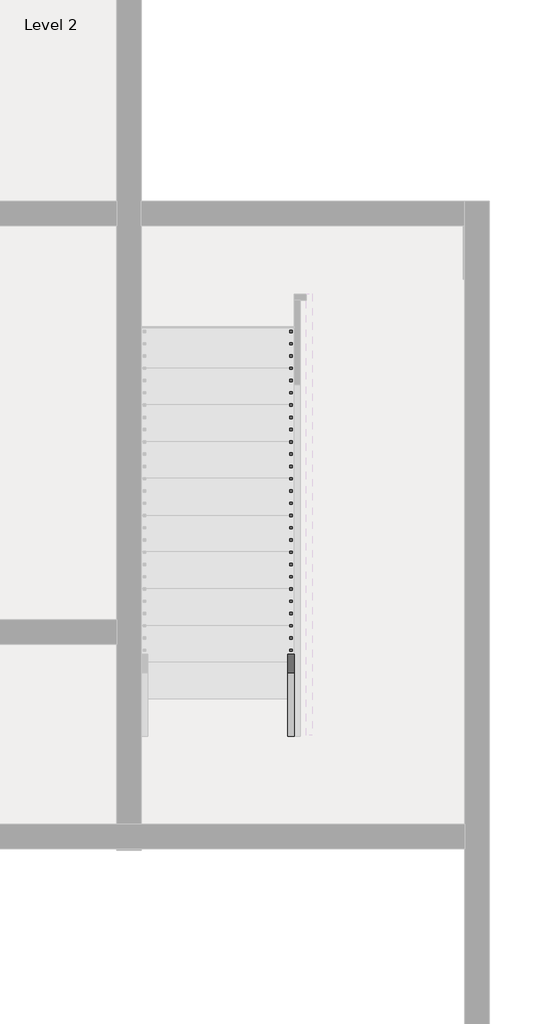
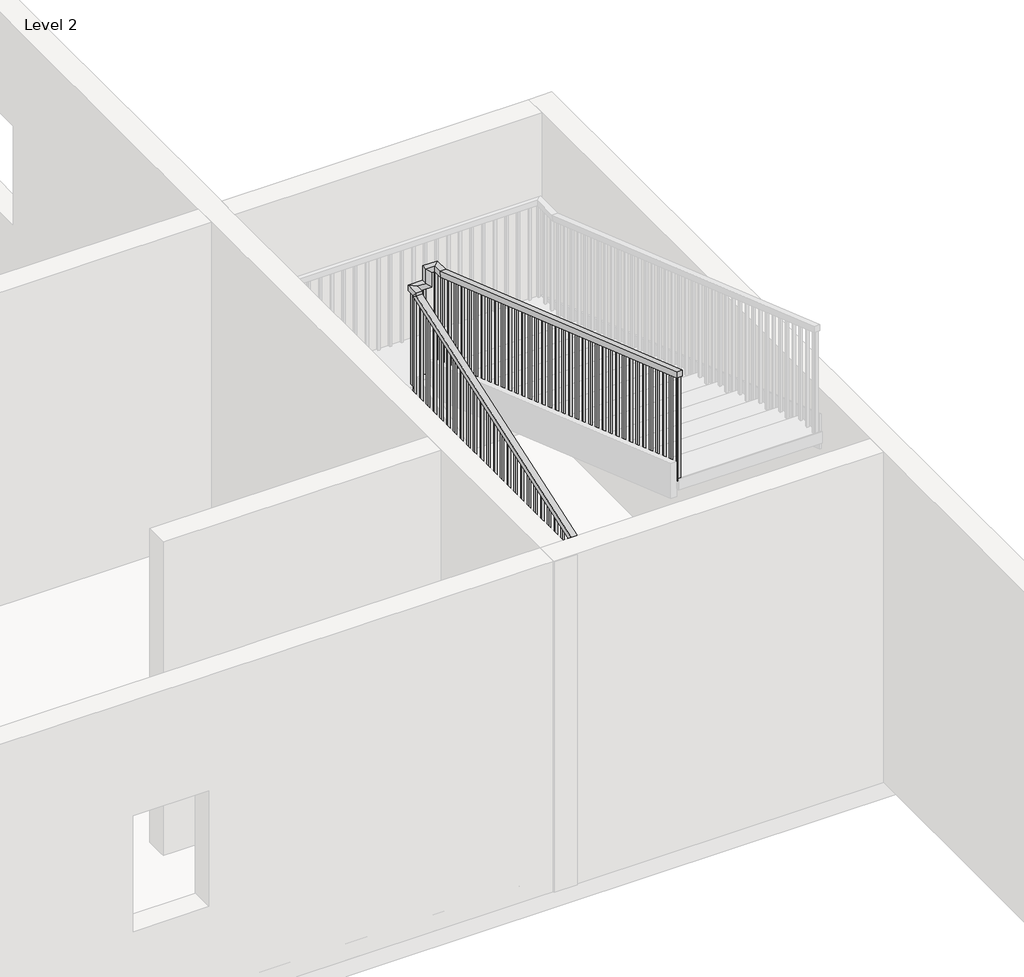
# One storey, part 6 of 14: 1 railing.
"""IFC4 building model written with IfcOpenShell, lengths in millimetres."""

from ifc_helpers import new_model, si_unit, frame, origin, place, context, project, spatial, polyline, outline, extrude, faceted_brep, element, save

model = new_model("IFC4")

# Units and contexts
model_context = context("Model", 3, world=origin())
ifc_project = project(units=[si_unit("LENGTHUNIT", "METRE", prefix="MILLI")], contexts=[model_context])

# Site, building, storey
site = spatial("IfcSite", under=ifc_project)
building = spatial("IfcBuilding", under=site)
storey = spatial("IfcBuildingStorey", under=building, Name="Level 2", Elevation=3048.0)

# Railing
placement = place(None, origin())
element("IfcRailing", 1, ObjectType="Handrail - Rectangular", at=placement, inside=storey, context=model_context, shape_type="SolidModel", body=[
    faceted_brep([(-2644.5381751, -9955.5916506, 4067.9076923), (-2644.5381751, -9955.5916506, 4014.1602476), (-2593.7381751, -9955.5916506, 4014.1602476), (-2593.7381751, -9955.5916506, 4067.9076923), (-2644.5381751, -6367.8416506, 5307.6687908), (-2644.5381751, -6317.0416506, 5271.4754856), (-2593.7381751, -6317.0416506, 5271.4754856), (-2593.7381751, -6367.8416506, 5307.6687908), (-2644.5381751, -6367.8416506, 5334.0), (-2644.5381751, -6317.0416506, 5283.2), (-2593.7381751, -6317.0416506, 5283.2), (-2593.7381751, -6367.8416506, 5334.0), (-2644.5381751, -6240.8416506, 5334.0), (-2644.5381751, -6240.8416506, 5283.2), (-2593.7381751, -6291.6416506, 5283.2), (-2593.7381751, -6291.6416506, 5334.0), (-2517.5381751, -6240.8416506, 5334.0), (-2466.7381751, -6240.8416506, 5283.2), (-2466.7381751, -6291.6416506, 5283.2), (-2517.5381751, -6291.6416506, 5334.0), (-2517.5381751, -6240.8416506, 5465.8846154), (-2466.7381751, -6240.8416506, 5415.0846154), (-2466.7381751, -6291.6416506, 5415.0846154), (-2517.5381751, -6291.6416506, 5465.8846154), (-2390.5381751, -6240.8416506, 5465.8846154), (-2390.5381751, -6240.8416506, 5415.0846154), (-2441.3381751, -6291.6416506, 5415.0846154), (-2441.3381751, -6291.6416506, 5465.8846154), (-2390.5381751, -6367.8416506, 5465.8846154), (-2390.5381751, -6376.3852679, 5415.0846154), (-2441.3381751, -6376.3852679, 5415.0846154), (-2441.3381751, -6367.8416506, 5465.8846154), (-2390.5381751, -9949.2416506, 6705.6), (-2441.3381751, -9949.2416506, 6705.6), (-2441.3381751, -9949.2416506, 6651.842594), (-2390.5381751, -9949.2416506, 6651.842594)], [[[0, 1, 2, 3]], [[1, 0, 4, 5]], [[2, 1, 5, 6]], [[3, 2, 6, 7]], [[0, 3, 7, 4]], [[5, 4, 8, 9]], [[6, 5, 9, 10]], [[7, 6, 10, 11]], [[4, 7, 11, 8]], [[9, 8, 12, 13]], [[10, 9, 13, 14]], [[11, 10, 14, 15]], [[8, 11, 15, 12]], [[13, 12, 16, 17]], [[14, 13, 17, 18]], [[15, 14, 18, 19]], [[12, 15, 19, 16]], [[17, 16, 20, 21]], [[18, 17, 21, 22]], [[19, 18, 22, 23]], [[16, 19, 23, 20]], [[21, 20, 24, 25]], [[22, 21, 25, 26]], [[23, 22, 26, 27]], [[20, 23, 27, 24]], [[25, 24, 28, 29]], [[26, 25, 29, 30]], [[27, 26, 30, 31]], [[24, 27, 31, 28]], [[32, 33, 34, 35]], [[29, 28, 32, 35]], [[30, 29, 35, 34]], [[31, 30, 34, 33]], [[28, 31, 33, 32]]]),
    extrude(outline(polyline([(-9933.3666506, 6646.3474017), (-9914.3166506, 6639.7531709), (-9914.3166506, 5685.6923077), (-9933.3666506, 5685.6923077), (-9933.3666506, 6646.3474017)])), frame((-2425.4631751, 0.0, 0.0), z_axis=(1.0, 0.0, 0.0), x_axis=(0.0, 1.0, 0.0)), (0.0, 0.0, 1.0), 19.05),
    extrude(outline(polyline([(-9831.7666506, 6611.1781709), (-9812.7166506, 6604.5839402), (-9812.7166506, 5685.6923077), (-9831.7666506, 5685.6923077), (-9831.7666506, 6611.1781709)])), frame((-2425.4631751, 0.0, 0.0), z_axis=(1.0, 0.0, 0.0), x_axis=(0.0, 1.0, 0.0)), (0.0, 0.0, 1.0), 19.05),
    extrude(outline(polyline([(-9730.1666506, 6576.0089402), (-9711.1166506, 6569.4147094), (-9711.1166506, 5685.6923077), (-9730.1666506, 5685.6923077), (-9730.1666506, 6576.0089402)])), frame((-2425.4631751, 0.0, 0.0), z_axis=(1.0, 0.0, 0.0), x_axis=(0.0, 1.0, 0.0)), (0.0, 0.0, 1.0), 19.05),
    extrude(outline(polyline([(-9628.5666506, 6540.8397094), (-9609.5166506, 6534.2454786), (-9609.5166506, 5580.1846154), (-9628.5666506, 5580.1846154), (-9628.5666506, 6540.8397094)])), frame((-2425.4631751, 0.0, 0.0), z_axis=(1.0, 0.0, 0.0), x_axis=(0.0, 1.0, 0.0)), (0.0, 0.0, 1.0), 19.05),
    extrude(outline(polyline([(-9526.9666506, 6505.6704786), (-9507.9166506, 6499.0762479), (-9507.9166506, 5580.1846154), (-9526.9666506, 5580.1846154), (-9526.9666506, 6505.6704786)])), frame((-2425.4631751, 0.0, 0.0), z_axis=(1.0, 0.0, 0.0), x_axis=(0.0, 1.0, 0.0)), (0.0, 0.0, 1.0), 19.05),
    extrude(outline(polyline([(-9425.3666506, 6470.5012479), (-9406.3166506, 6463.9070171), (-9406.3166506, 5580.1846154), (-9425.3666506, 5580.1846154), (-9425.3666506, 6470.5012479)])), frame((-2425.4631751, 0.0, 0.0), z_axis=(1.0, 0.0, 0.0), x_axis=(0.0, 1.0, 0.0)), (0.0, 0.0, 1.0), 19.05),
    extrude(outline(polyline([(-9323.7666506, 6435.3320171), (-9304.7166506, 6428.7377863), (-9304.7166506, 5474.6769231), (-9323.7666506, 5474.6769231), (-9323.7666506, 6435.3320171)])), frame((-2425.4631751, 0.0, 0.0), z_axis=(1.0, 0.0, 0.0), x_axis=(0.0, 1.0, 0.0)), (0.0, 0.0, 1.0), 19.05),
    extrude(outline(polyline([(-9222.1666506, 6400.1627863), (-9203.1166506, 6393.5685556), (-9203.1166506, 5474.6769231), (-9222.1666506, 5474.6769231), (-9222.1666506, 6400.1627863)])), frame((-2425.4631751, 0.0, 0.0), z_axis=(1.0, 0.0, 0.0), x_axis=(0.0, 1.0, 0.0)), (0.0, 0.0, 1.0), 19.05),
    extrude(outline(polyline([(-9120.5666506, 6364.9935556), (-9101.5166506, 6358.3993248), (-9101.5166506, 5474.6769231), (-9120.5666506, 5474.6769231), (-9120.5666506, 6364.9935556)])), frame((-2425.4631751, 0.0, 0.0), z_axis=(1.0, 0.0, 0.0), x_axis=(0.0, 1.0, 0.0)), (0.0, 0.0, 1.0), 19.05),
    extrude(outline(polyline([(-9018.9666506, 6329.8243248), (-8999.9166506, 6323.230094), (-8999.9166506, 5369.1692308), (-9018.9666506, 5369.1692308), (-9018.9666506, 6329.8243248)])), frame((-2425.4631751, 0.0, 0.0), z_axis=(1.0, 0.0, 0.0), x_axis=(0.0, 1.0, 0.0)), (0.0, 0.0, 1.0), 19.05),
    extrude(outline(polyline([(-8917.3666506, 6294.655094), (-8898.3166506, 6288.0608632), (-8898.3166506, 5369.1692308), (-8917.3666506, 5369.1692308), (-8917.3666506, 6294.655094)])), frame((-2425.4631751, 0.0, 0.0), z_axis=(1.0, 0.0, 0.0), x_axis=(0.0, 1.0, 0.0)), (0.0, 0.0, 1.0), 19.05),
    extrude(outline(polyline([(-8815.7666506, 6259.4858632), (-8796.7166506, 6252.8916325), (-8796.7166506, 5369.1692308), (-8815.7666506, 5369.1692308), (-8815.7666506, 6259.4858632)])), frame((-2425.4631751, 0.0, 0.0), z_axis=(1.0, 0.0, 0.0), x_axis=(0.0, 1.0, 0.0)), (0.0, 0.0, 1.0), 19.05),
    extrude(outline(polyline([(-8714.1666506, 6224.3166325), (-8695.1166506, 6217.7224017), (-8695.1166506, 5263.6615385), (-8714.1666506, 5263.6615385), (-8714.1666506, 6224.3166325)])), frame((-2425.4631751, 0.0, 0.0), z_axis=(1.0, 0.0, 0.0), x_axis=(0.0, 1.0, 0.0)), (0.0, 0.0, 1.0), 19.05),
    extrude(outline(polyline([(-8612.5666506, 6189.1474017), (-8593.5166506, 6182.5531709), (-8593.5166506, 5263.6615385), (-8612.5666506, 5263.6615385), (-8612.5666506, 6189.1474017)])), frame((-2425.4631751, 0.0, 0.0), z_axis=(1.0, 0.0, 0.0), x_axis=(0.0, 1.0, 0.0)), (0.0, 0.0, 1.0), 19.05),
    extrude(outline(polyline([(-8510.9666506, 6153.9781709), (-8491.9166506, 6147.3839402), (-8491.9166506, 5263.6615385), (-8510.9666506, 5263.6615385), (-8510.9666506, 6153.9781709)])), frame((-2425.4631751, 0.0, 0.0), z_axis=(1.0, 0.0, 0.0), x_axis=(0.0, 1.0, 0.0)), (0.0, 0.0, 1.0), 19.05),
    extrude(outline(polyline([(-8409.3666506, 6118.8089402), (-8390.3166506, 6112.2147094), (-8390.3166506, 5158.1538462), (-8409.3666506, 5158.1538462), (-8409.3666506, 6118.8089402)])), frame((-2425.4631751, 0.0, 0.0), z_axis=(1.0, 0.0, 0.0), x_axis=(0.0, 1.0, 0.0)), (0.0, 0.0, 1.0), 19.05),
    extrude(outline(polyline([(-8307.7666506, 6083.6397094), (-8288.7166506, 6077.0454786), (-8288.7166506, 5158.1538462), (-8307.7666506, 5158.1538462), (-8307.7666506, 6083.6397094)])), frame((-2425.4631751, 0.0, 0.0), z_axis=(1.0, 0.0, 0.0), x_axis=(0.0, 1.0, 0.0)), (0.0, 0.0, 1.0), 19.05),
    extrude(outline(polyline([(-8206.1666506, 6048.4704786), (-8187.1166506, 6041.8762479), (-8187.1166506, 5158.1538462), (-8206.1666506, 5158.1538462), (-8206.1666506, 6048.4704786)])), frame((-2425.4631751, 0.0, 0.0), z_axis=(1.0, 0.0, 0.0), x_axis=(0.0, 1.0, 0.0)), (0.0, 0.0, 1.0), 19.05),
    extrude(outline(polyline([(-8104.5666506, 6013.3012479), (-8085.5166506, 6006.7070171), (-8085.5166506, 5052.6461538), (-8104.5666506, 5052.6461538), (-8104.5666506, 6013.3012479)])), frame((-2425.4631751, 0.0, 0.0), z_axis=(1.0, 0.0, 0.0), x_axis=(0.0, 1.0, 0.0)), (0.0, 0.0, 1.0), 19.05),
    extrude(outline(polyline([(-8002.9666506, 5978.1320171), (-7983.9166506, 5971.5377863), (-7983.9166506, 5052.6461538), (-8002.9666506, 5052.6461538), (-8002.9666506, 5978.1320171)])), frame((-2425.4631751, 0.0, 0.0), z_axis=(1.0, 0.0, 0.0), x_axis=(0.0, 1.0, 0.0)), (0.0, 0.0, 1.0), 19.05),
    extrude(outline(polyline([(-7901.3666506, 5942.9627863), (-7882.3166506, 5936.3685556), (-7882.3166506, 5052.6461538), (-7901.3666506, 5052.6461538), (-7901.3666506, 5942.9627863)])), frame((-2425.4631751, 0.0, 0.0), z_axis=(1.0, 0.0, 0.0), x_axis=(0.0, 1.0, 0.0)), (0.0, 0.0, 1.0), 19.05),
    extrude(outline(polyline([(-7799.7666506, 5907.7935556), (-7780.7166506, 5901.1993248), (-7780.7166506, 4947.1384615), (-7799.7666506, 4947.1384615), (-7799.7666506, 5907.7935556)])), frame((-2425.4631751, 0.0, 0.0), z_axis=(1.0, 0.0, 0.0), x_axis=(0.0, 1.0, 0.0)), (0.0, 0.0, 1.0), 19.05),
    extrude(outline(polyline([(-7698.1666506, 5872.6243248), (-7679.1166506, 5866.030094), (-7679.1166506, 4947.1384615), (-7698.1666506, 4947.1384615), (-7698.1666506, 5872.6243248)])), frame((-2425.4631751, 0.0, 0.0), z_axis=(1.0, 0.0, 0.0), x_axis=(0.0, 1.0, 0.0)), (0.0, 0.0, 1.0), 19.05),
    extrude(outline(polyline([(-7596.5666506, 5837.455094), (-7577.5166506, 5830.8608632), (-7577.5166506, 4947.1384615), (-7596.5666506, 4947.1384615), (-7596.5666506, 5837.455094)])), frame((-2425.4631751, 0.0, 0.0), z_axis=(1.0, 0.0, 0.0), x_axis=(0.0, 1.0, 0.0)), (0.0, 0.0, 1.0), 19.05),
    extrude(outline(polyline([(-7494.9666506, 5802.2858632), (-7475.9166506, 5795.6916325), (-7475.9166506, 4841.6307692), (-7494.9666506, 4841.6307692), (-7494.9666506, 5802.2858632)])), frame((-2425.4631751, 0.0, 0.0), z_axis=(1.0, 0.0, 0.0), x_axis=(0.0, 1.0, 0.0)), (0.0, 0.0, 1.0), 19.05),
    extrude(outline(polyline([(-7393.3666506, 5767.1166325), (-7374.3166506, 5760.5224017), (-7374.3166506, 4841.6307692), (-7393.3666506, 4841.6307692), (-7393.3666506, 5767.1166325)])), frame((-2425.4631751, 0.0, 0.0), z_axis=(1.0, 0.0, 0.0), x_axis=(0.0, 1.0, 0.0)), (0.0, 0.0, 1.0), 19.05),
    extrude(outline(polyline([(-7291.7666506, 5731.9474017), (-7272.7166506, 5725.3531709), (-7272.7166506, 4841.6307692), (-7291.7666506, 4841.6307692), (-7291.7666506, 5731.9474017)])), frame((-2425.4631751, 0.0, 0.0), z_axis=(1.0, 0.0, 0.0), x_axis=(0.0, 1.0, 0.0)), (0.0, 0.0, 1.0), 19.05),
    extrude(outline(polyline([(-7190.1666506, 5696.7781709), (-7171.1166506, 5690.1839402), (-7171.1166506, 4736.1230769), (-7190.1666506, 4736.1230769), (-7190.1666506, 5696.7781709)])), frame((-2425.4631751, 0.0, 0.0), z_axis=(1.0, 0.0, 0.0), x_axis=(0.0, 1.0, 0.0)), (0.0, 0.0, 1.0), 19.05),
    extrude(outline(polyline([(-7088.5666506, 5661.6089402), (-7069.5166506, 5655.0147094), (-7069.5166506, 4736.1230769), (-7088.5666506, 4736.1230769), (-7088.5666506, 5661.6089402)])), frame((-2425.4631751, 0.0, 0.0), z_axis=(1.0, 0.0, 0.0), x_axis=(0.0, 1.0, 0.0)), (0.0, 0.0, 1.0), 19.05),
    extrude(outline(polyline([(-6986.9666506, 5626.4397094), (-6967.9166506, 5619.8454786), (-6967.9166506, 4736.1230769), (-6986.9666506, 4736.1230769), (-6986.9666506, 5626.4397094)])), frame((-2425.4631751, 0.0, 0.0), z_axis=(1.0, 0.0, 0.0), x_axis=(0.0, 1.0, 0.0)), (0.0, 0.0, 1.0), 19.05),
    extrude(outline(polyline([(-6885.3666506, 5591.2704786), (-6866.3166506, 5584.6762479), (-6866.3166506, 4630.6153846), (-6885.3666506, 4630.6153846), (-6885.3666506, 5591.2704786)])), frame((-2425.4631751, 0.0, 0.0), z_axis=(1.0, 0.0, 0.0), x_axis=(0.0, 1.0, 0.0)), (0.0, 0.0, 1.0), 19.05),
    extrude(outline(polyline([(-6783.7666506, 5556.1012479), (-6764.7166506, 5549.5070171), (-6764.7166506, 4630.6153846), (-6783.7666506, 4630.6153846), (-6783.7666506, 5556.1012479)])), frame((-2425.4631751, 0.0, 0.0), z_axis=(1.0, 0.0, 0.0), x_axis=(0.0, 1.0, 0.0)), (0.0, 0.0, 1.0), 19.05),
    extrude(outline(polyline([(-6682.1666506, 5520.9320171), (-6663.1166506, 5514.3377863), (-6663.1166506, 4630.6153846), (-6682.1666506, 4630.6153846), (-6682.1666506, 5520.9320171)])), frame((-2425.4631751, 0.0, 0.0), z_axis=(1.0, 0.0, 0.0), x_axis=(0.0, 1.0, 0.0)), (0.0, 0.0, 1.0), 19.05),
    extrude(outline(polyline([(-6580.5666506, 5485.7627863), (-6561.5166506, 5479.1685556), (-6561.5166506, 4525.1076923), (-6580.5666506, 4525.1076923), (-6580.5666506, 5485.7627863)])), frame((-2425.4631751, 0.0, 0.0), z_axis=(1.0, 0.0, 0.0), x_axis=(0.0, 1.0, 0.0)), (0.0, 0.0, 1.0), 19.05),
    extrude(outline(polyline([(-6478.9666506, 5450.5935556), (-6459.9166506, 5443.9993248), (-6459.9166506, 4525.1076923), (-6478.9666506, 4525.1076923), (-6478.9666506, 5450.5935556)])), frame((-2425.4631751, 0.0, 0.0), z_axis=(1.0, 0.0, 0.0), x_axis=(0.0, 1.0, 0.0)), (0.0, 0.0, 1.0), 19.05),
    extrude(outline(polyline([(-6377.3666506, 5415.4243248), (-6358.3166506, 5408.830094), (-6358.3166506, 4525.1076923), (-6377.3666506, 4525.1076923), (-6377.3666506, 5415.4243248)])), frame((-2425.4631751, 0.0, 0.0), z_axis=(1.0, 0.0, 0.0), x_axis=(0.0, 1.0, 0.0)), (0.0, 0.0, 1.0), 19.05),
    extrude(outline(polyline([(-2527.0631751, -6275.7666506), (-2527.0631751, -6256.7166506), (-2508.0131751, -6256.7166506), (-2508.0131751, -6275.7666506), (-2527.0631751, -6275.7666506)])), frame((0.0, 0.0, 4419.6), z_axis=(0.0, 0.0, 1.0), x_axis=(1.0, 0.0, 0.0)), (0.0, 0.0, 1.0), 863.6),
    extrude(outline(polyline([(-2609.6131751, -6307.5166506), (-2628.6631751, -6307.5166506), (-2628.6631751, -6288.4666506), (-2609.6131751, -6288.4666506), (-2609.6131751, -6307.5166506)])), frame((0.0, 0.0, 4314.0923077), z_axis=(0.0, 0.0, 1.0), x_axis=(1.0, 0.0, 0.0)), (0.0, 0.0, 1.0), 969.1076923),
    extrude(outline(polyline([(-6409.1166506, 5239.6586078), (-6390.0666506, 5246.2414101), (-6390.0666506, 4314.0923077), (-6409.1166506, 4314.0923077), (-6409.1166506, 5239.6586078)])), frame((-2628.6631751, 0.0, 0.0), z_axis=(1.0, 0.0, 0.0), x_axis=(0.0, 1.0, 0.0)), (0.0, 0.0, 1.0), 19.05),
    extrude(outline(polyline([(-6510.7166506, 5204.5503289), (-6491.6666506, 5211.1331312), (-6491.6666506, 4314.0923077), (-6510.7166506, 4314.0923077), (-6510.7166506, 5204.5503289)])), frame((-2628.6631751, 0.0, 0.0), z_axis=(1.0, 0.0, 0.0), x_axis=(0.0, 1.0, 0.0)), (0.0, 0.0, 1.0), 19.05),
    extrude(outline(polyline([(-6612.3166506, 5169.44205), (-6593.2666506, 5176.0248523), (-6593.2666506, 4208.5846154), (-6612.3166506, 4208.5846154), (-6612.3166506, 5169.44205)])), frame((-2628.6631751, 0.0, 0.0), z_axis=(1.0, 0.0, 0.0), x_axis=(0.0, 1.0, 0.0)), (0.0, 0.0, 1.0), 19.05),
    extrude(outline(polyline([(-6713.9166506, 5134.3337711), (-6694.8666506, 5140.9165734), (-6694.8666506, 4208.5846154), (-6713.9166506, 4208.5846154), (-6713.9166506, 5134.3337711)])), frame((-2628.6631751, 0.0, 0.0), z_axis=(1.0, 0.0, 0.0), x_axis=(0.0, 1.0, 0.0)), (0.0, 0.0, 1.0), 19.05),
    extrude(outline(polyline([(-6815.5166506, 5099.2254922), (-6796.4666506, 5105.8082945), (-6796.4666506, 4208.5846154), (-6815.5166506, 4208.5846154), (-6815.5166506, 5099.2254922)])), frame((-2628.6631751, 0.0, 0.0), z_axis=(1.0, 0.0, 0.0), x_axis=(0.0, 1.0, 0.0)), (0.0, 0.0, 1.0), 19.05),
    extrude(outline(polyline([(-6917.1166506, 5064.1172133), (-6898.0666506, 5070.7000156), (-6898.0666506, 4103.0769231), (-6917.1166506, 4103.0769231), (-6917.1166506, 5064.1172133)])), frame((-2628.6631751, 0.0, 0.0), z_axis=(1.0, 0.0, 0.0), x_axis=(0.0, 1.0, 0.0)), (0.0, 0.0, 1.0), 19.05),
    extrude(outline(polyline([(-7018.7166506, 5029.0089344), (-6999.6666506, 5035.5917367), (-6999.6666506, 4103.0769231), (-7018.7166506, 4103.0769231), (-7018.7166506, 5029.0089344)])), frame((-2628.6631751, 0.0, 0.0), z_axis=(1.0, 0.0, 0.0), x_axis=(0.0, 1.0, 0.0)), (0.0, 0.0, 1.0), 19.05),
    extrude(outline(polyline([(-7120.3166506, 4993.9006556), (-7101.2666506, 5000.4834578), (-7101.2666506, 4103.0769231), (-7120.3166506, 4103.0769231), (-7120.3166506, 4993.9006556)])), frame((-2628.6631751, 0.0, 0.0), z_axis=(1.0, 0.0, 0.0), x_axis=(0.0, 1.0, 0.0)), (0.0, 0.0, 1.0), 19.05),
    extrude(outline(polyline([(-7221.9166506, 4958.7923767), (-7202.8666506, 4965.3751789), (-7202.8666506, 3997.5692308), (-7221.9166506, 3997.5692308), (-7221.9166506, 4958.7923767)])), frame((-2628.6631751, 0.0, 0.0), z_axis=(1.0, 0.0, 0.0), x_axis=(0.0, 1.0, 0.0)), (0.0, 0.0, 1.0), 19.05),
    extrude(outline(polyline([(-7323.5166506, 4923.6840978), (-7304.4666506, 4930.2669001), (-7304.4666506, 3997.5692308), (-7323.5166506, 3997.5692308), (-7323.5166506, 4923.6840978)])), frame((-2628.6631751, 0.0, 0.0), z_axis=(1.0, 0.0, 0.0), x_axis=(0.0, 1.0, 0.0)), (0.0, 0.0, 1.0), 19.05),
    extrude(outline(polyline([(-7425.1166506, 4888.5758189), (-7406.0666506, 4895.1586212), (-7406.0666506, 3997.5692308), (-7425.1166506, 3997.5692308), (-7425.1166506, 4888.5758189)])), frame((-2628.6631751, 0.0, 0.0), z_axis=(1.0, 0.0, 0.0), x_axis=(0.0, 1.0, 0.0)), (0.0, 0.0, 1.0), 19.05),
    extrude(outline(polyline([(-7526.7166506, 4853.46754), (-7507.6666506, 4860.0503423), (-7507.6666506, 3892.0615385), (-7526.7166506, 3892.0615385), (-7526.7166506, 4853.46754)])), frame((-2628.6631751, 0.0, 0.0), z_axis=(1.0, 0.0, 0.0), x_axis=(0.0, 1.0, 0.0)), (0.0, 0.0, 1.0), 19.05),
    extrude(outline(polyline([(-7628.3166506, 4818.3592611), (-7609.2666506, 4824.9420634), (-7609.2666506, 3892.0615385), (-7628.3166506, 3892.0615385), (-7628.3166506, 4818.3592611)])), frame((-2628.6631751, 0.0, 0.0), z_axis=(1.0, 0.0, 0.0), x_axis=(0.0, 1.0, 0.0)), (0.0, 0.0, 1.0), 19.05),
    extrude(outline(polyline([(-7729.9166506, 4783.2509822), (-7710.8666506, 4789.8337845), (-7710.8666506, 3892.0615385), (-7729.9166506, 3892.0615385), (-7729.9166506, 4783.2509822)])), frame((-2628.6631751, 0.0, 0.0), z_axis=(1.0, 0.0, 0.0), x_axis=(0.0, 1.0, 0.0)), (0.0, 0.0, 1.0), 19.05),
    extrude(outline(polyline([(-7831.5166506, 4748.1427033), (-7812.4666506, 4754.7255056), (-7812.4666506, 3786.5538462), (-7831.5166506, 3786.5538462), (-7831.5166506, 4748.1427033)])), frame((-2628.6631751, 0.0, 0.0), z_axis=(1.0, 0.0, 0.0), x_axis=(0.0, 1.0, 0.0)), (0.0, 0.0, 1.0), 19.05),
    extrude(outline(polyline([(-7933.1166506, 4713.0344244), (-7914.0666506, 4719.6172267), (-7914.0666506, 3786.5538462), (-7933.1166506, 3786.5538462), (-7933.1166506, 4713.0344244)])), frame((-2628.6631751, 0.0, 0.0), z_axis=(1.0, 0.0, 0.0), x_axis=(0.0, 1.0, 0.0)), (0.0, 0.0, 1.0), 19.05),
    extrude(outline(polyline([(-8034.7166506, 4677.9261455), (-8015.6666506, 4684.5089478), (-8015.6666506, 3786.5538462), (-8034.7166506, 3786.5538462), (-8034.7166506, 4677.9261455)])), frame((-2628.6631751, 0.0, 0.0), z_axis=(1.0, 0.0, 0.0), x_axis=(0.0, 1.0, 0.0)), (0.0, 0.0, 1.0), 19.05),
    extrude(outline(polyline([(-8136.3166506, 4642.8178666), (-8117.2666506, 4649.4006689), (-8117.2666506, 3681.0461538), (-8136.3166506, 3681.0461538), (-8136.3166506, 4642.8178666)])), frame((-2628.6631751, 0.0, 0.0), z_axis=(1.0, 0.0, 0.0), x_axis=(0.0, 1.0, 0.0)), (0.0, 0.0, 1.0), 19.05),
    extrude(outline(polyline([(-8237.9166506, 4607.7095877), (-8218.8666506, 4614.29239), (-8218.8666506, 3681.0461538), (-8237.9166506, 3681.0461538), (-8237.9166506, 4607.7095877)])), frame((-2628.6631751, 0.0, 0.0), z_axis=(1.0, 0.0, 0.0), x_axis=(0.0, 1.0, 0.0)), (0.0, 0.0, 1.0), 19.05),
    extrude(outline(polyline([(-8339.5166506, 4572.6013088), (-8320.4666506, 4579.1841111), (-8320.4666506, 3681.0461538), (-8339.5166506, 3681.0461538), (-8339.5166506, 4572.6013088)])), frame((-2628.6631751, 0.0, 0.0), z_axis=(1.0, 0.0, 0.0), x_axis=(0.0, 1.0, 0.0)), (0.0, 0.0, 1.0), 19.05),
    extrude(outline(polyline([(-8441.1166506, 4537.4930299), (-8422.0666506, 4544.0758322), (-8422.0666506, 3575.5384615), (-8441.1166506, 3575.5384615), (-8441.1166506, 4537.4930299)])), frame((-2628.6631751, 0.0, 0.0), z_axis=(1.0, 0.0, 0.0), x_axis=(0.0, 1.0, 0.0)), (0.0, 0.0, 1.0), 19.05),
    extrude(outline(polyline([(-8542.7166506, 4502.384751), (-8523.6666506, 4508.9675533), (-8523.6666506, 3575.5384615), (-8542.7166506, 3575.5384615), (-8542.7166506, 4502.384751)])), frame((-2628.6631751, 0.0, 0.0), z_axis=(1.0, 0.0, 0.0), x_axis=(0.0, 1.0, 0.0)), (0.0, 0.0, 1.0), 19.05),
    extrude(outline(polyline([(-8644.3166506, 4467.2764721), (-8625.2666506, 4473.8592744), (-8625.2666506, 3575.5384615), (-8644.3166506, 3575.5384615), (-8644.3166506, 4467.2764721)])), frame((-2628.6631751, 0.0, 0.0), z_axis=(1.0, 0.0, 0.0), x_axis=(0.0, 1.0, 0.0)), (0.0, 0.0, 1.0), 19.05),
    extrude(outline(polyline([(-8745.9166506, 4432.1681932), (-8726.8666506, 4438.7509955), (-8726.8666506, 3470.0307692), (-8745.9166506, 3470.0307692), (-8745.9166506, 4432.1681932)])), frame((-2628.6631751, 0.0, 0.0), z_axis=(1.0, 0.0, 0.0), x_axis=(0.0, 1.0, 0.0)), (0.0, 0.0, 1.0), 19.05),
    extrude(outline(polyline([(-8847.5166506, 4397.0599143), (-8828.4666506, 4403.6427166), (-8828.4666506, 3470.0307692), (-8847.5166506, 3470.0307692), (-8847.5166506, 4397.0599143)])), frame((-2628.6631751, 0.0, 0.0), z_axis=(1.0, 0.0, 0.0), x_axis=(0.0, 1.0, 0.0)), (0.0, 0.0, 1.0), 19.05),
    extrude(outline(polyline([(-8949.1166506, 4361.9516354), (-8930.0666506, 4368.5344377), (-8930.0666506, 3470.0307692), (-8949.1166506, 3470.0307692), (-8949.1166506, 4361.9516354)])), frame((-2628.6631751, 0.0, 0.0), z_axis=(1.0, 0.0, 0.0), x_axis=(0.0, 1.0, 0.0)), (0.0, 0.0, 1.0), 19.05),
    extrude(outline(polyline([(-9050.7166506, 4326.8433565), (-9031.6666506, 4333.4261588), (-9031.6666506, 3364.5230769), (-9050.7166506, 3364.5230769), (-9050.7166506, 4326.8433565)])), frame((-2628.6631751, 0.0, 0.0), z_axis=(1.0, 0.0, 0.0), x_axis=(0.0, 1.0, 0.0)), (0.0, 0.0, 1.0), 19.05),
    extrude(outline(polyline([(-9152.3166506, 4291.7350776), (-9133.2666506, 4298.3178799), (-9133.2666506, 3364.5230769), (-9152.3166506, 3364.5230769), (-9152.3166506, 4291.7350776)])), frame((-2628.6631751, 0.0, 0.0), z_axis=(1.0, 0.0, 0.0), x_axis=(0.0, 1.0, 0.0)), (0.0, 0.0, 1.0), 19.05),
    extrude(outline(polyline([(-9253.9166506, 4256.6267987), (-9234.8666506, 4263.209601), (-9234.8666506, 3364.5230769), (-9253.9166506, 3364.5230769), (-9253.9166506, 4256.6267987)])), frame((-2628.6631751, 0.0, 0.0), z_axis=(1.0, 0.0, 0.0), x_axis=(0.0, 1.0, 0.0)), (0.0, 0.0, 1.0), 19.05),
    extrude(outline(polyline([(-9355.5166506, 4221.5185198), (-9336.4666506, 4228.1013221), (-9336.4666506, 3259.0153846), (-9355.5166506, 3259.0153846), (-9355.5166506, 4221.5185198)])), frame((-2628.6631751, 0.0, 0.0), z_axis=(1.0, 0.0, 0.0), x_axis=(0.0, 1.0, 0.0)), (0.0, 0.0, 1.0), 19.05),
    extrude(outline(polyline([(-9457.1166506, 4186.4102409), (-9438.0666506, 4192.9930432), (-9438.0666506, 3259.0153846), (-9457.1166506, 3259.0153846), (-9457.1166506, 4186.4102409)])), frame((-2628.6631751, 0.0, 0.0), z_axis=(1.0, 0.0, 0.0), x_axis=(0.0, 1.0, 0.0)), (0.0, 0.0, 1.0), 19.05),
    extrude(outline(polyline([(-9558.7166506, 4151.301962), (-9539.6666506, 4157.8847643), (-9539.6666506, 3259.0153846), (-9558.7166506, 3259.0153846), (-9558.7166506, 4151.301962)])), frame((-2628.6631751, 0.0, 0.0), z_axis=(1.0, 0.0, 0.0), x_axis=(0.0, 1.0, 0.0)), (0.0, 0.0, 1.0), 19.05),
    extrude(outline(polyline([(-9660.3166506, 4116.1936831), (-9641.2666506, 4122.7764854), (-9641.2666506, 3153.5076923), (-9660.3166506, 3153.5076923), (-9660.3166506, 4116.1936831)])), frame((-2628.6631751, 0.0, 0.0), z_axis=(1.0, 0.0, 0.0), x_axis=(0.0, 1.0, 0.0)), (0.0, 0.0, 1.0), 19.05),
    extrude(outline(polyline([(-9761.9166506, 4081.0854043), (-9742.8666506, 4087.6682065), (-9742.8666506, 3153.5076923), (-9761.9166506, 3153.5076923), (-9761.9166506, 4081.0854043)])), frame((-2628.6631751, 0.0, 0.0), z_axis=(1.0, 0.0, 0.0), x_axis=(0.0, 1.0, 0.0)), (0.0, 0.0, 1.0), 19.05),
    extrude(outline(polyline([(-9863.5166506, 4045.9771254), (-9844.4666506, 4052.5599277), (-9844.4666506, 3153.5076923), (-9863.5166506, 3153.5076923), (-9863.5166506, 4045.9771254)])), frame((-2628.6631751, 0.0, 0.0), z_axis=(1.0, 0.0, 0.0), x_axis=(0.0, 1.0, 0.0)), (0.0, 0.0, 1.0), 19.05),
    extrude(outline(polyline([(-2425.4631751, -6275.7666506), (-2425.4631751, -6256.7166506), (-2406.4131751, -6256.7166506), (-2406.4131751, -6275.7666506), (-2425.4631751, -6275.7666506)])), frame((0.0, 0.0, 4419.6), z_axis=(0.0, 0.0, 1.0), x_axis=(1.0, 0.0, 0.0)), (0.0, 0.0, 1.0), 995.4846154),
    extrude(outline(polyline([(-2609.6131751, -6275.7666506), (-2628.6631751, -6275.7666506), (-2628.6631751, -6256.7166506), (-2609.6131751, -6256.7166506), (-2609.6131751, -6275.7666506)])), frame((0.0, 0.0, 4419.6), z_axis=(0.0, 0.0, 1.0), x_axis=(1.0, 0.0, 0.0)), (0.0, 0.0, 1.0), 863.6),
    extrude(outline(polyline([(-9949.2416506, 6651.842594), (-9930.1916506, 6645.2483632), (-9930.1916506, 5685.6923077), (-9949.2416506, 5685.6923077), (-9949.2416506, 6651.842594)])), frame((-2425.4631751, 0.0, 0.0), z_axis=(1.0, 0.0, 0.0), x_axis=(0.0, 1.0, 0.0)), (0.0, 0.0, 1.0), 19.05),
    extrude(outline(polyline([(-9955.5916506, 4014.1602476), (-9936.5416506, 4020.7430499), (-9936.5416506, 3153.5076923), (-9955.5916506, 3153.5076923), (-9955.5916506, 4014.1602476)])), frame((-2628.6631751, 0.0, 0.0), z_axis=(1.0, 0.0, 0.0), x_axis=(0.0, 1.0, 0.0)), (0.0, 0.0, 1.0), 19.05),
])

save(model, "model.ifc")

# Revit data of these elements
# Type "Handrail - Rectangular"
#   Assembly Code = "C2010400"
#   built-in parameter 1008612 = 0.0416667 (stored number, unit not read)
#   built-in parameter 1008611 = 0.0416667 (stored number, unit not read)
#   built-in parameter 1008609 = 0.333333 (stored number, unit not read)
#   built-in parameter 1008604 = 0.166667 (stored number, unit not read)
#   built-in parameter 1008603 = 0.166667 (stored number, unit not read)
#   Railing Height = 3' - 0"
#   built-in parameter 1008630 = 2
#   built-in parameter 1008610 = 2
#   built-in parameter 1008618 = Baluster - Square : 3/4"
# Element 1 (IfcRailing, "Handrail - Rectangular")
#   Phase Created = New Construction
